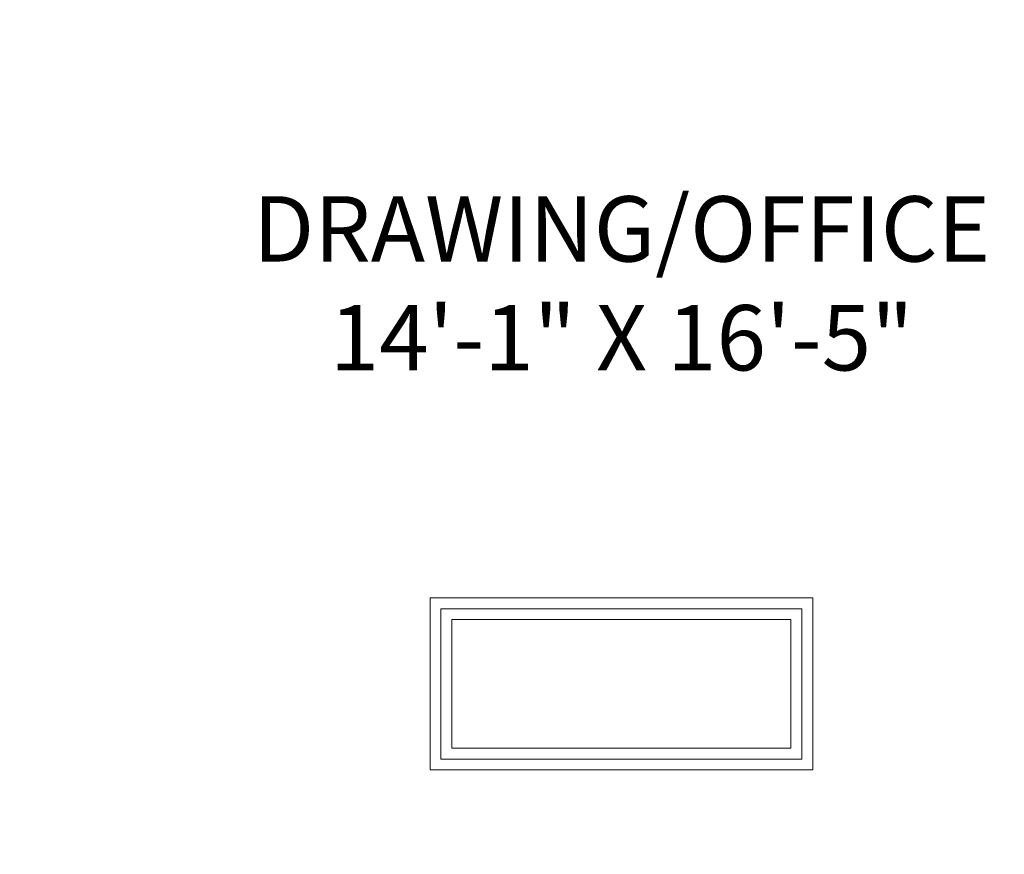
# Model space of a CAD drawing. Units: inches. Extents: x -466983 to 1020, y 324 to 318697.
# Tile 31 of 97: x 817 to 908, y 658 to 734. Entities that reach past the tile are written whole.
import ezdxf

# ---------------------------------------------------------------- set-up
doc = ezdxf.new("R2010")
doc.units = ezdxf.units.IN
doc.header["$MEASUREMENT"] = 0
for name, color, linetype, lineweight in [('A-ANNO-DIMS', 2, 'Continuous', 18), ('A-AREA-IDEN', 7, 'Continuous', 25), ('A-FLOR-PATT', 252, 'Continuous', 13), ('A-FURN', 8, 'Continuous', 18)]:
    doc.layers.add(name, color=color, linetype=linetype, lineweight=lineweight)
doc.styles.get("Standard").update_dxf_attribs({"font": 'arial.ttf'})
doc.dimstyles.get("Standard").update_dxf_attribs({"dimtxt": 6, "dimasz": 4, "dimexe": 3, "dimexo": 3, "dimgap": 0.09, "dimtad": 0, "dimtih": 1, "dimtoh": 1, "dimdec": 1, "dimzin": 0, "dimdsep": 46, "dimlunit": 3, "dimtxsty": 'Standard', "dimcen": 0.09, "dimadec": 0, "dimazin": 0, "dimtfac": 1, "dimtdec": 1, "dimtofl": 0, "dimtmove": 0, "dimatfit": 3, "dimfxl": 1, "dimtolj": 1, "dimtzin": 0, "dimarcsym": 0})

# ---------------------------------------------------------------- blocks, each defined once
blk = doc.blocks.new('RUG')
for points in [[(0, 35.137), (15.803, 35.137), (15.803, 0), (0, 0)], [(1, 34.137), (14.803, 34.137), (14.803, 1), (1, 1)], [(2, 33.137), (13.803, 33.137), (13.803, 2), (2, 2)]]:
    blk.add_lwpolyline(points, close=True)
blk = doc.blocks.new('*D91')
at = {"layer": 'A-ANNO-DIMS', "color": 0, "lineweight": -2, "transparency": 16777216}
for p, q in [((938.253, 802.547), (920.07, 802.547)), ((923.07, 798.547), (923.07, 745.132)), ((923.07, 685.328), (923.07, 738.743)), ((938.253, 681.328), (920.07, 681.328))]:
    blk.add_line(p, q, dxfattribs=at)
at = {"layer": 'A-ANNO-DIMS', "color": 0, "transparency": 16777216}
for points in [[(922.404, 798.547), (923.737, 798.547), (923.07, 802.547)], [(922.404, 685.328), (923.737, 685.328), (923.07, 681.328)]]:
    blk.add_solid(points, dxfattribs=at)
at = {"layer": 'Defpoints', "color": 0, "transparency": 16777216}
for p in [(941.253, 802.547), (923.07, 681.328), (941.253, 681.328)]:
    blk.add_point(p, dxfattribs=at)
at = {"layer": 'A-ANNO-DIMS', "color": 0, "transparency": 16777216, "insert": (923.07, 741.937), "char_height": 6, "attachment_point": 5}
blk.add_mtext('\\A1;4-SEATER SOFA 121', dxfattribs=at)

msp = doc.modelspace()

# ---------------------------------------------------------------- hatches: boundary and pattern name
at = {"layer": 'A-FLOR-PATT', "transparency": 33554572}
h = msp.add_hatch(dxfattribs=at)
h.set_pattern_fill('ANSI37', color=256, scale=30)
h.set_pattern_definition([(45, (-1212.4137, -290.035), (-2.6516504, 2.6516504), []), (135, (-1212.4137, -290.035), (-2.6516504, -2.6516504), [])])
h.paths.add_polyline_path([(901.806, 1075.938), (900.614, 1075.938), (900.614, 1065.386), (899.391, 1065.386), (898.091, 1065.386), (892.836, 1058.71, -0.258377), (892.188, 1058.351), (879.985, 1058.351, -0.20177), (879.438, 1058.581), (874.081, 1065.386), (872.781, 1065.386), (871.558, 1065.386), (871.558, 1075.938), (813.806, 1075.938), (813.806, 1044.792), (832.395, 1044.792, -0.394795), (848.66, 1028.536), (848.66, 1009.938), (901.806, 1009.938), (901.806, 1015.938), (901.306, 1015.938), (871.306, 1015.938), (871.306, 1017.25), (871.334, 1017.25, -0.401453), (901.306, 1045.938), (901.806, 1045.938)])
edge = h.paths.add_edge_path(flags=16)
edge.add_line((847.773, 1068.949), (847.773, 1073.709))
edge.add_arc((849.227, 1073.709), 1.454, 90, 180, ccw=False)
edge.add_line((849.227, 1075.163), (864.492, 1075.163))
edge.add_arc((864.492, 1073.709), 1.454, 0, 90, ccw=False)
edge.add_line((865.946, 1073.709), (865.946, 1069.004))
edge.add_arc((832.645, 1068.976), 33.301, -20.61234, 0.04725, ccw=False)
edge.add_ellipse((856.859, 1058.48), major_axis=(0, 10.213), ratio=0.685919, start_angle=100.00884, end_angle=259.99116, ccw=False)
edge.add_arc((881.074, 1068.976), 33.301, 180.04725, 200.61234, ccw=False)
h.paths.add_polyline_path([(853.146, 1066.482), (853.146, 1066.453), (853.146, 1066.453, 0.433107), (852.917, 1066.685), (852.917, 1066.453), (853.146, 1066.453), (853.146, 1066.482), (853.088, 1066.612, 0.697939), (852.7, 1066.453), (852.7, 1066.453), (852.7, 1066.482), (852.917, 1067.001), (852.917, 1066.685, -0.396254)], flags=0)
h.paths.add_polyline_path([(861.019, 1066.482), (861.019, 1066.453), (861.019, 1066.453, 0.416404), (860.802, 1066.685), (860.802, 1066.453), (861.019, 1066.453), (861.019, 1066.482), (860.967, 1066.605, 0.713344), (860.573, 1066.453), (860.573, 1066.453), (860.573, 1066.482), (860.802, 1067.001), (860.802, 1066.685, -0.379973)], flags=0)
edge = h.paths.add_edge_path(flags=0)
edge.add_spline(control_points=[(861.13, 1065.785), (861.466, 1065.248), (861.613, 1065.016), (861.983, 1064.374), (862.192, 1063.944), (862.561, 1063.039), (862.721, 1062.563), (862.987, 1061.578), (863.092, 1061.069), (863.245, 1060.031), (863.293, 1059.503), (863.329, 1058.441), (863.318, 1057.908), (863.237, 1056.852), (863.166, 1056.329), (862.97, 1055.308), (862.843, 1054.81), (862.537, 1053.852), (862.357, 1053.393), (861.951, 1052.525), (861.725, 1052.117), (861.233, 1051.362), (860.967, 1051.016), (860.405, 1050.395), (860.108, 1050.12), (859.494, 1049.646), (859.176, 1049.448), (858.528, 1049.13), (858.197, 1049.011), (857.531, 1048.852), (857.196, 1048.812), (856.525, 1048.812), (856.189, 1048.852), (855.524, 1049.01), (855.193, 1049.129), (854.545, 1049.447), (854.227, 1049.645), (853.612, 1050.118), (853.316, 1050.393), (852.753, 1051.014), (852.487, 1051.36), (851.995, 1052.114), (851.769, 1052.523), (851.363, 1053.39), (851.183, 1053.85), (850.877, 1054.807), (850.75, 1055.305), (850.553, 1056.326), (850.483, 1056.849), (850.401, 1057.905), (850.39, 1058.438), (850.426, 1059.5), (850.473, 1060.028), (850.626, 1061.066), (850.732, 1061.575), (850.997, 1062.561), (851.157, 1063.036), (851.525, 1063.942), (851.734, 1064.371), (852.106, 1065.016), (852.254, 1065.25), (852.608, 1065.733)], knot_values=[3.915332, 3.915332, 3.915332, 3.915332, 4.013468, 4.013468, 4.175532, 4.175532, 4.337596, 4.337596, 4.49966, 4.49966, 4.661724, 4.661724, 4.823788, 4.823788, 4.985852, 4.985852, 5.147916, 5.147916, 5.30998, 5.30998, 5.472044, 5.472044, 5.634109, 5.634109, 5.796173, 5.796173, 5.958237, 5.958237, 6.120301, 6.120301, 6.282365, 6.282365, 6.444429, 6.444429, 6.606493, 6.606493, 6.768557, 6.768557, 6.930621, 6.930621, 7.092685, 7.092685, 7.254749, 7.254749, 7.416813, 7.416813, 7.578878, 7.578878, 7.740942, 7.740942, 7.903006, 7.903006, 8.06507, 8.06507, 8.227134, 8.227134, 8.389198, 8.389198, 8.551262, 8.551262, 8.65037, 8.65037, 8.65037, 8.65037], degree=3, periodic=0)
edge.add_line((852.642, 1065.785), (861.13, 1065.785))
edge = h.paths.add_edge_path(flags=0)
edge.add_ellipse((856.85, 1057.743), major_axis=(0, 7.792), ratio=0.687861, start_angle=0, end_angle=360)
h.paths.add_polyline_path([(848.863, 1069.389), (848.863, 1073.96, -0.414214), (849.954, 1075.051), (863.765, 1075.051, -0.414214), (864.856, 1073.96), (864.856, 1069.389, -0.388936), (864.524, 1069.027, -0.043561), (849.195, 1069.027, -0.388936)], flags=0)
h.paths.add_polyline_path([(853.101, 1068.112, -1), (852.677, 1068.112, -1)], flags=0)
edge = h.paths.add_edge_path(flags=0)
edge.add_ellipse((856.859, 1057.338), major_axis=(0, 2.207), ratio=0.657164, start_angle=0, end_angle=360)
h.paths.add_polyline_path([(861.041, 1068.112, -1), (860.618, 1068.112, -1)], flags=0)
edge = h.paths.add_edge_path()
edge.add_line((573.954, 1057.341), (573.954, 1075.938))
edge.add_line((573.954, 1075.938), (558.731, 1075.938))
edge.add_line((558.731, 1075.938), (558.731, 1065.386))
edge.add_line((558.731, 1065.386), (557.507, 1065.386))
edge.add_line((557.507, 1065.386), (556.207, 1065.386))
edge.add_line((556.207, 1065.386), (550.952, 1058.71))
edge.add_arc((550.304, 1059.116), 0.765, 270, 327.94832, ccw=False)
edge.add_line((550.304, 1058.351), (538.101, 1058.351))
edge.add_arc((538.101, 1059.116), 0.765, 224.3704, 270, ccw=False)
edge.add_line((537.555, 1058.581), (532.198, 1065.386))
edge.add_line((532.198, 1065.386), (530.898, 1065.386))
edge.add_line((530.898, 1065.386), (529.674, 1065.386))
edge.add_line((529.674, 1065.386), (529.674, 1075.938))
edge.add_line((529.674, 1075.938), (520.806, 1075.938))
edge.add_line((520.806, 1075.938), (520.806, 1045.938))
edge.add_line((520.806, 1045.938), (521.306, 1045.938))
edge.add_arc((521.306, 1015.938), 30, 2.50749, 90, ccw=False)
edge.add_line((551.277, 1017.25), (551.306, 1017.25))
edge.add_line((551.306, 1017.25), (551.306, 1015.938))
edge.add_line((551.306, 1015.938), (520.806, 1015.938))
edge.add_line((520.806, 1015.938), (520.806, 1009.938))
edge.add_line((520.806, 1009.938), (559.191, 1010.402))
edge.add_arc((559.191, 1011.856), 1.454, 180, 270, ccw=False)
edge.add_line((557.737, 1011.856), (557.737, 1016.561))
edge.add_arc((591.039, 1016.589), 33.301, 159.38766, 180.04725, ccw=False)
edge.add_ellipse((566.824, 1027.085), major_axis=(0, 10.213), ratio=0.685919, start_angle=280.00884, end_angle=439.99116, ccw=False)
edge.add_arc((542.609, 1016.589), 33.301, 0.04725, 20.61234, ccw=False)
edge.add_line((575.91, 1016.616), (575.91, 1011.856))
edge.add_arc((574.456, 1011.856), 1.454, -90, 0, ccw=False)
edge.add_line((574.456, 1010.402), (608.806, 1009.938))
edge.add_line((608.806, 1009.938), (608.806, 1041.086))
edge.add_line((608.806, 1041.086), (590.218, 1041.086))
edge.add_arc((590.775, 1057.907), 16.831, 181.92775, 268.10321, ccw=False)
edge = h.paths.add_edge_path()
edge.add_ellipse((494.244, 583.62), major_axis=(0, 10.213), ratio=0.685919, start_angle=280.00884, end_angle=439.99116, ccw=False)
edge.add_arc((470.03, 573.124), 33.301, 0.04725, 20.61234, ccw=False)
edge.add_line((503.331, 573.152), (503.331, 568.392))
edge.add_arc((501.877, 568.392), 1.454, -90, 0, ccw=False)
edge.add_line((501.877, 566.938), (539.806, 566.938))
edge.add_line((539.806, 566.938), (539.806, 572.938))
edge.add_line((539.806, 572.938), (539.306, 572.938))
edge.add_line((539.306, 572.938), (509.306, 572.938))
edge.add_line((509.306, 572.938), (509.306, 574.25))
edge.add_line((509.306, 574.25), (509.334, 574.25))
edge.add_arc((539.306, 572.938), 30, 90, 177.49251, ccw=False)
edge.add_line((539.306, 602.938), (539.806, 602.938))
edge.add_line((539.806, 602.938), (539.806, 626.938))
edge.add_line((539.806, 626.938), (531.772, 626.938))
edge.add_line((531.772, 626.938), (531.772, 616.386))
edge.add_line((531.772, 616.386), (530.548, 616.386))
edge.add_line((530.548, 616.386), (529.249, 616.386))
edge.add_line((529.249, 616.386), (523.711, 609.351))
edge.add_line((523.711, 609.351), (510.777, 609.351))
edge.add_line((510.777, 609.351), (505.239, 616.386))
edge.add_line((505.239, 616.386), (503.939, 616.386))
edge.add_line((503.939, 616.386), (502.715, 616.386))
edge.add_line((502.715, 616.386), (502.715, 626.938))
edge.add_line((502.715, 626.938), (481.698, 626.938))
edge.add_line((481.698, 626.938), (481.698, 610.995))
edge.add_arc((467.27, 611.473), 14.436, 271.92775, 358.10321, ccw=False)
edge.add_line((467.756, 597.045), (451.806, 597.045))
edge.add_line((451.806, 597.045), (451.806, 584.404))
edge.add_line((451.806, 584.404), (451.806, 566.938))
edge.add_line((451.806, 566.938), (486.612, 566.938))
edge.add_arc((486.612, 568.392), 1.454, 180, 270, ccw=False)
edge.add_line((485.158, 568.392), (485.158, 573.097))
edge.add_arc((518.459, 573.124), 33.301, 159.38766, 180.04725, ccw=False)
h.paths.add_polyline_path([(836.261, 1020.733), (879.89, 1020.733), (879.89, 1039.39), (836.261, 1039.39)], flags=25)
h.paths.add_polyline_path([(549.985, 1036.749), (593.614, 1036.749), (593.614, 1055.407), (549.985, 1055.407)], flags=24)
h.paths.add_polyline_path([(475.123, 595.596), (518.752, 595.596), (518.752, 614.253), (475.123, 614.253)], flags=24)

# ---------------------------------------------------------------- block references
at = {"layer": 'A-FURN', "rotation": 270.0000000000005}
msp.add_blockref('RUG', (855.005, 681.274), dxfattribs=at)

# ---------------------------------------------------------------- texts
at = {"layer": 'A-AREA-IDEN', "insert": (757.806, 718.167), "char_height": 6, "attachment_point": 1}
msp.add_mtext_dynamic_manual_height_columns('\\pxqc;{\\fArial|b1|i0|c0|p34;DRAWING/OFFICE\\P14\'-1" X 16\'-5"}', width=229.55829, gutter_width=1, heights=[0], dxfattribs=at)

# ---------------------------------------------------------------- dimensions: what is measured, and where the dimension line sits
at = {"layer": 'A-ANNO-DIMS'}
dim = msp.add_linear_dim(base=(923.07, 681.328), p1=(941.253, 802.547), p2=(941.253, 681.328), angle=270, text='4-SEATER SOFA <>', dimstyle='Standard', override={"dimdec": 0, "dimlfac": 1, "dimrnd": 0, "dimzin": 0, "dimdsep": 46, "dimlunit": 2}, dxfattribs=at)
dim.commit()
dim.dimension.update_dxf_attribs({"geometry": '*D91', "text_midpoint": (923.07, 741.937)})

doc.saveas('drawing.dxf')
